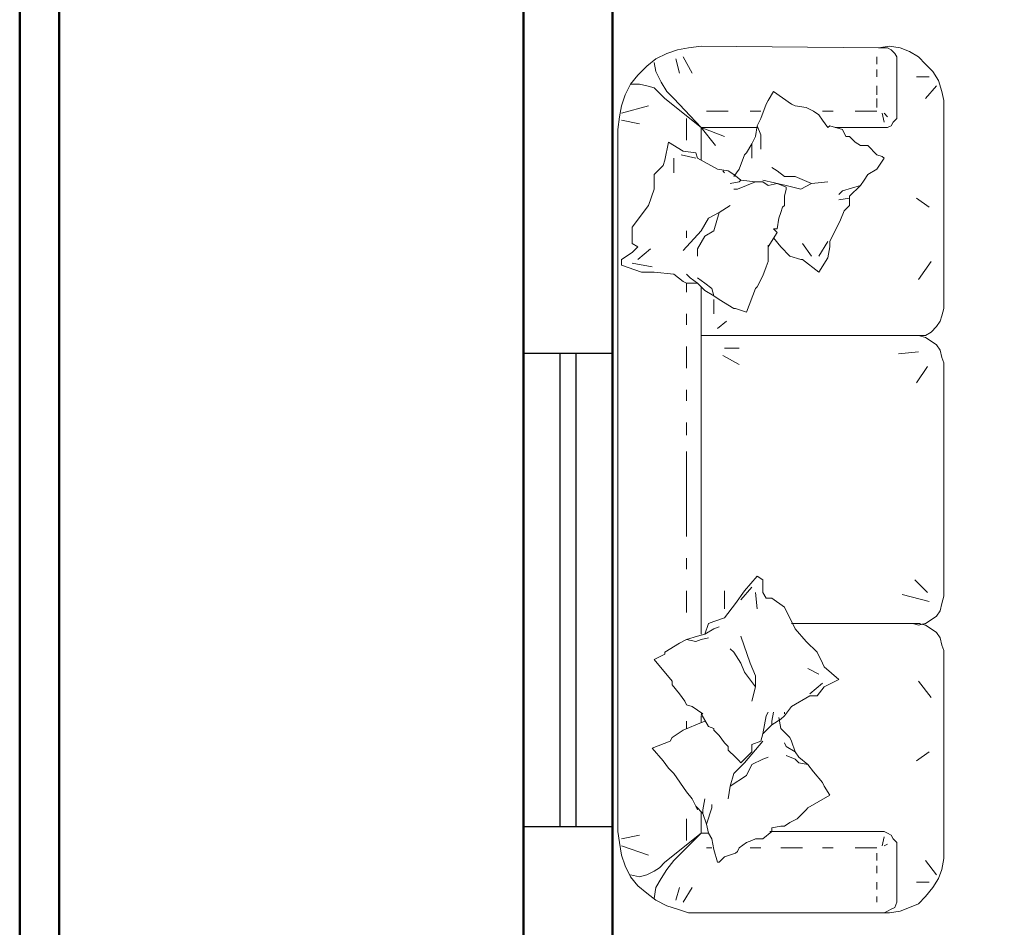
# Model space of a CAD drawing. Units: inches. Extents: x -466983 to 1020, y 324 to 318697.
# Tile 42 of 97: x 392 to 491, y 881 to 973. Entities that reach past the tile are written whole.
import ezdxf

# ---------------------------------------------------------------- set-up
doc = ezdxf.new("R2010")
doc.units = ezdxf.units.IN
doc.header["$MEASUREMENT"] = 0
for name, color, linetype, lineweight in [('A-FLOR-PATT', 252, 'Continuous', 13), ('A-FURN', 8, 'Continuous', 18), ('A-GLAZ', 4, 'Continuous', 25), ('A-WALL', 7, 'Continuous', 50)]:
    doc.layers.add(name, color=color, linetype=linetype, lineweight=lineweight)

# ---------------------------------------------------------------- blocks, each defined once
blk = doc.blocks.new('Window 4 ft')
for p, q in [((1224.69, 893.769), (1233.69, 893.769)), ((1224.69, 845.769), (1224.69, 893.769)), ((1228.39, 845.769), (1228.39, 893.769)), ((1229.99, 893.769), (1229.99, 845.769)), ((1233.69, 893.769), (1233.69, 845.769)), ((1233.69, 845.769), (1224.69, 845.769))]:
    blk.add_line(p, q)
blk = doc.blocks.new('sofa-36')
at = {"linetype": 'ByBlock'}
for p, q in [((-0.105, 0.895), (-0.08, 0.9)), ((-0.08, 0.9), (-0.105, 0.895)), ((-0.08, 0.9), (0.495, 0.9)), ((0.495, 0.9), (-0.08, 0.9)), ((0.495, 0.9), (0.515, 0.895)), ((0.515, 0.895), (0.495, 0.9)), ((0.63, 0.895), (0.645, 0.9)), ((0.63, 0.895), (0.645, 0.9)), ((0.645, 0.9), (0.87, 0.9)), ((0.87, 0.9), (0.645, 0.9)), ((0.87, 0.9), (1.29, 0.9)), ((1.29, 0.9), (0.87, 0.9)), ((1.29, 0.9), (1.31, 0.895)), ((1.31, 0.895), (1.29, 0.9)), ((1.425, 0.895), (1.44, 0.9)), ((1.425, 0.895), (1.44, 0.9)), ((1.44, 0.9), (2.015, 0.9)), ((2.015, 0.9), (1.44, 0.9)), ((2.015, 0.9), (2.045, 0.895)), ((2.045, 0.895), (2.015, 0.9)), ((-0.18, 0.85), (-0.16, 0.87)), ((-0.16, 0.87), (-0.18, 0.85)), ((-0.16, 0.87), (-0.135, 0.885)), ((-0.135, 0.885), (-0.16, 0.87)), ((-0.135, 0.885), (-0.105, 0.895)), ((-0.105, 0.895), (-0.135, 0.885)), ((-0.085, 0.85), (-0.12, 0.88)), ((0.515, 0.895), (0.53, 0.89)), ((0.53, 0.89), (0.515, 0.895)), ((0.53, 0.89), (0.545, 0.88)), ((0.545, 0.88), (0.53, 0.89)), ((0.545, 0.88), (0.56, 0.865)), ((0.56, 0.865), (0.545, 0.88)), ((0.585, 0.865), (0.595, 0.88)), ((0.585, 0.865), (0.595, 0.88)), ((0.595, 0.88), (0.61, 0.89)), ((0.595, 0.88), (0.61, 0.89)), ((0.61, 0.89), (0.63, 0.895)), ((0.61, 0.89), (0.63, 0.895)), ((1.31, 0.895), (1.33, 0.89)), ((1.33, 0.89), (1.31, 0.895)), ((1.33, 0.89), (1.345, 0.88)), ((1.345, 0.88), (1.33, 0.89)), ((1.345, 0.88), (1.355, 0.865)), ((1.355, 0.865), (1.345, 0.88)), ((1.38, 0.865), (1.39, 0.88)), ((1.38, 0.865), (1.39, 0.88)), ((1.39, 0.88), (1.405, 0.89)), ((1.39, 0.88), (1.405, 0.89)), ((1.405, 0.89), (1.425, 0.895)), ((1.405, 0.89), (1.425, 0.895)), ((2.02, 0.85), (2.06, 0.88)), ((2.045, 0.895), (2.07, 0.885)), ((2.07, 0.885), (2.045, 0.895)), ((2.07, 0.885), (2.095, 0.87)), ((2.095, 0.87), (2.07, 0.885)), ((2.095, 0.87), (2.12, 0.85)), ((2.12, 0.85), (2.095, 0.87)), ((-0.2, 0.83), (-0.18, 0.85)), ((-0.18, 0.85), (-0.2, 0.83)), ((-0.145, 0.825), (-0.145, 0.86)), ((0.19, 0.825), (0.215, 0.86)), ((0.415, 0.83), (0.365, 0.865)), ((0.56, 0.865), (0.57, 0.85)), ((0.57, 0.85), (0.56, 0.865)), ((0.57, 0.83), (0.575, 0.85)), ((0.57, 0.85), (0.57, 0.83)), ((0.57, 0.83), (0.57, 0.85)), ((0.57, 0.83), (0.575, 0.85)), ((0.575, 0.85), (0.585, 0.865)), ((0.575, 0.85), (0.585, 0.865)), ((0.655, 0.855), (0.7, 0.825)), ((1.28, 0.855), (1.245, 0.82)), ((1.305, 0.86), (1.285, 0.785)), ((1.355, 0.865), (1.365, 0.85)), ((1.365, 0.85), (1.355, 0.865)), ((1.365, 0.85), (1.3675, 0.84)), ((1.37, 0.83), (1.365, 0.85)), ((1.365, 0.83), (1.37, 0.85)), ((1.3675, 0.84), (1.37, 0.85)), ((1.37, 0.85), (1.38, 0.865)), ((1.37, 0.85), (1.38, 0.865)), ((1.525, 0.83), (1.57, 0.865)), ((1.745, 0.825), (1.72, 0.86)), ((2.08, 0.825), (2.08, 0.86)), ((2.12, 0.85), (2.14, 0.83)), ((2.14, 0.83), (2.12, 0.85)), ((-0.215, 0.805), (-0.2, 0.83)), ((-0.2, 0.83), (-0.215, 0.805)), ((0.57, 0.835), (0.57, 0.23)), ((0.57, 0.815), (0.57, 0.83)), ((0.57, 0.815), (0.57, 0.83)), ((0.615, 0.83), (0.62, 0.775)), ((1.365, 0.835), (1.365, 0.48)), ((1.365, 0.815), (1.37, 0.83)), ((1.365, 0.815), (1.365, 0.83)), ((2.14, 0.83), (2.15, 0.805)), ((2.15, 0.805), (2.14, 0.83)), ((-0.225, 0.78), (-0.215, 0.805)), ((-0.215, 0.805), (-0.225, 0.78)), ((2.15, 0.805), (2.16, 0.78)), ((2.16, 0.78), (2.15, 0.805)), ((-0.23, 0.75), (-0.225, 0.78)), ((-0.225, 0.78), (-0.23, 0.75)), ((-0.22, 0.755), (-0.21, 0.765)), ((-0.21, 0.765), (-0.2, 0.77)), ((-0.2, 0.77), (-0.19, 0.77)), ((-0.19, 0.77), (-0.175, 0.77)), ((-0.175, 0.77), (-0.055, 0.77)), ((-0.055, 0.77), (-0.04, 0.77)), ((-0.04, 0.77), (-0.03, 0.77)), ((-0.03, 0.77), (-0.02, 0.76)), ((1.96, 0.76), (1.97, 0.77)), ((1.97, 0.77), (1.98, 0.77)), ((1.98, 0.77), (1.99, 0.77)), ((1.99, 0.77), (2.115, 0.77)), ((2.115, 0.77), (2.125, 0.77)), ((2.125, 0.77), (2.135, 0.77)), ((2.135, 0.77), (2.15, 0.765)), ((2.15, 0.765), (2.155, 0.755)), ((2.16, 0.78), (2.165, 0.75)), ((2.165, 0.75), (2.16, 0.78)), ((-0.225, 0.72), (-0.23, 0.75)), ((-0.23, 0.75), (-0.225, 0.72)), ((-0.225, 0.745), (-0.22, 0.755)), ((-0.225, 0.735), (-0.225, 0.745)), ((-0.225, 0.72), (-0.225, 0.735)), ((-0.045, 0.735), (-0.035, 0.745)), ((-0.045, 0.73), (-0.02, 0.735)), ((-0.02, 0.76), (-0.01, 0.755)), ((-0.01, 0.755), (-0.005, 0.745)), ((-0.005, 0.745), (-0.005, 0.735)), ((-0.005, 0.735), (-0.005, 0.72)), ((0.08, 0.735), (0.075, 0.73)), ((0.11, 0.715), (0.08, 0.735)), ((1.94, 0.735), (1.945, 0.745)), ((1.94, 0.72), (1.94, 0.735)), ((1.945, 0.745), (1.95, 0.755)), ((1.95, 0.755), (1.96, 0.76)), ((1.98, 0.73), (1.955, 0.735)), ((1.98, 0.735), (1.975, 0.745)), ((2.155, 0.755), (2.16, 0.745)), ((2.16, 0.745), (2.165, 0.735)), ((2.165, 0.75), (2.165, 0.72)), ((2.165, 0.72), (2.165, 0.75)), ((2.165, 0.735), (2.165, 0.72)), ((-0.23, 0.23), (-0.225, 0.72)), ((-0.23, 0.23), (-0.225, 0.72)), ((-0.2, 0.715), (-0.18, 0.715)), ((-0.165, 0.715), (-0.145, 0.715)), ((-0.12, 0.715), (-0.095, 0.715)), ((-0.085, 0.715), (-0.06, 0.715)), ((-0.05, 0.715), (-0.05, 0.655)), ((-0.005, 0.72), (-0.005, 0.6)), ((0.07, 0.715), (0.045, 0.69)), ((0.075, 0.73), (0.07, 0.715)), ((0.125, 0.69), (0.11, 0.715)), ((1.94, 0.42), (1.94, 0.72)), ((1.985, 0.715), (1.985, 0.655)), ((2.02, 0.715), (2, 0.715)), ((2.055, 0.715), (2.035, 0.715)), ((2.1, 0.715), (2.08, 0.715)), ((2.135, 0.715), (2.12, 0.715)), ((2.165, 0.72), (2.165, 0.23)), ((2.165, 0.72), (2.165, 0.23)), ((0.045, 0.69), (0.045, 0.68)), ((0.045, 0.68), (0.045, 0.67)), ((0.14, 0.68), (0.125, 0.69)), ((0.155, 0.67), (0.14, 0.68)), ((0.035, 0.655), (0.02, 0.64)), ((0.045, 0.67), (0.035, 0.655)), ((0.155, 0.67), (0.17, 0.62)), ((0.185, 0.64), (0.155, 0.67)), ((0.02, 0.63), (0, 0.62)), ((0.02, 0.64), (0.02, 0.63)), ((0.185, 0.64), (0.21, 0.64)), ((0.19, 0.64), (0.185, 0.64)), ((0.195, 0.61), (0.19, 0.64)), ((0.21, 0.64), (0.225, 0.625)), ((0, 0.62), (-0.01, 0.585)), ((0.17, 0.62), (0.18, 0.61)), ((0.225, 0.625), (0.25, 0.615)), ((0.235, 0.62), (0.235, 0.62)), ((0.25, 0.615), (0.31, 0.585)), ((1.52, 0.61), (1.485, 0.57)), ((1.54, 0.57), (1.52, 0.61)), ((-0.05, 0.595), (-0.05, 0.565)), ((-0.005, 0.58), (-0.025, 0.565)), ((-0.01, 0.585), (-0.005, 0.58)), ((0.15, 0.535), (0.145, 0.58)), ((0.31, 0.585), (0.325, 0.585)), ((0.35, 0.555), (0.31, 0.58)), ((0.325, 0.585), (0.355, 0.58)), ((0.355, 0.58), (0.395, 0.555)), ((1.815, 0.57), (1.84, 0.585)), ((1.84, 0.585), (1.875, 0.525)), ((1.985, 0.595), (1.985, 0.565)), ((-0.04, 0.555), (-0.05, 0.54)), ((-0.025, 0.565), (-0.04, 0.555)), ((0.395, 0.555), (0.36, 0.51)), ((1.445, 0.55), (1.415, 0.52)), ((1.475, 0.565), (1.445, 0.55)), ((1.485, 0.57), (1.475, 0.565)), ((1.505, 0.555), (1.49, 0.525)), ((1.53, 0.565), (1.56, 0.53)), ((1.565, 0.55), (1.54, 0.57)), ((1.565, 0.53), (1.565, 0.55)), ((1.775, 0.54), (1.805, 0.565)), ((1.805, 0.565), (1.815, 0.57)), ((-0.06, 0.52), (-0.065, 0.49)), ((-0.05, 0.54), (-0.06, 0.52)), ((0.15, 0.535), (0.13, 0.49)), ((0.165, 0.505), (0.15, 0.535)), ((0.35, 0.535), (0.315, 0.51)), ((1.415, 0.52), (1.38, 0.49)), ((1.595, 0.48), (1.565, 0.53)), ((1.735, 0.5), (1.755, 0.525)), ((1.755, 0.525), (1.75, 0.5)), ((1.755, 0.525), (1.775, 0.54)), ((1.875, 0.525), (1.88, 0.52)), ((1.88, 0.52), (1.905, 0.495)), ((-0.065, 0.49), (-0.07, 0.48)), ((0.13, 0.49), (0.13, 0.46)), ((0.155, 0.465), (0.165, 0.505)), ((0.36, 0.505), (0.35, 0.475)), ((0.36, 0.51), (0.36, 0.505)), ((1.38, 0.49), (1.32, 0.46)), ((1.72, 0.49), (1.69, 0.48)), ((1.705, 0.465), (1.72, 0.49)), ((1.72, 0.49), (1.735, 0.5)), ((1.74, 0.49), (1.73, 0.465)), ((1.75, 0.5), (1.74, 0.49)), ((1.905, 0.495), (1.915, 0.475)), ((1.985, 0.45), (1.985, 0.51)), ((-0.07, 0.48), (-0.105, 0.43)), ((0.14, 0.4), (0.155, 0.465)), ((0.16, 0.465), (0.15, 0.44)), ((0.165, 0.465), (0.16, 0.465)), ((0.185, 0.46), (0.165, 0.465)), ((0.35, 0.475), (0.325, 0.45)), ((1.62, 0.46), (1.595, 0.48)), ((1.68, 0.475), (1.655, 0.45)), ((1.69, 0.48), (1.68, 0.475)), ((1.695, 0.46), (1.705, 0.465)), ((1.915, 0.475), (1.925, 0.46)), ((0.115, 0.44), (0.105, 0.425)), ((0.13, 0.46), (0.115, 0.44)), ((0.15, 0.44), (0.155, 0.415)), ((0.21, 0.46), (0.185, 0.46)), ((0.215, 0.455), (0.21, 0.46)), ((0.23, 0.45), (0.215, 0.455)), ((0.245, 0.445), (0.23, 0.45)), ((0.275, 0.44), (0.245, 0.445)), ((0.275, 0.43), (0.275, 0.44)), ((0.285, 0.44), (0.275, 0.43)), ((0.325, 0.415), (0.285, 0.44)), ((0.325, 0.45), (0.3, 0.43)), ((1.32, 0.46), (1.295, 0.425)), ((1.615, 0.46), (1.61, 0.46)), ((1.63, 0.45), (1.62, 0.46)), ((1.655, 0.45), (1.625, 0.445)), ((1.645, 0.425), (1.63, 0.45)), ((1.925, 0.46), (1.925, 0.45)), ((1.925, 0.45), (1.93, 0.425)), ((-0.105, 0.43), (-0.08, 0.415)), ((-0.08, 0.415), (-0.07, 0.41)), ((-0.07, 0.41), (-0.03, 0.395)), ((0.155, 0.415), (0.145, 0.4)), ((0.32, 0.415), (0.325, 0.415)), ((0.355, 0.415), (0.32, 0.415)), ((0.365, 0.415), (0.355, 0.415)), ((0.38, 0.41), (0.365, 0.415)), ((0.405, 0.4), (0.38, 0.41)), ((1.295, 0.41), (1.28, 0.4)), ((1.295, 0.425), (1.295, 0.41)), ((1.61, 0.43), (1.635, 0.425)), ((1.62, 0.41), (1.61, 0.415)), ((1.67, 0.4), (1.62, 0.41)), ((1.635, 0.425), (1.645, 0.425)), ((1.645, 0.425), (1.67, 0.4)), ((1.74, 0.4), (1.735, 0.415)), ((1.93, 0.425), (1.94, 0.425)), ((1.94, 0.425), (1.96, 0.4)), ((-0.05, 0.365), (-0.05, 0.395)), ((-0.03, 0.395), (-0.01, 0.385)), ((-0.01, 0.385), (0.015, 0.395)), ((-0.01, 0.385), (0.02, 0.38)), ((-0.005, 0.385), (-0.005, 0.23)), ((0.015, 0.395), (0.03, 0.395)), ((0.03, 0.395), (0.055, 0.395)), ((0.145, 0.4), (0.145, 0.38)), ((0.435, 0.385), (0.405, 0.4)), ((0.44, 0.38), (0.435, 0.385)), ((1.245, 0.4), (1.235, 0.385)), ((1.235, 0.385), (1.275, 0.35)), ((1.28, 0.4), (1.245, 0.4)), ((1.28, 0.38), (1.325, 0.385)), ((1.67, 0.4), (1.69, 0.395)), ((1.69, 0.4), (1.75, 0.35)), ((1.69, 0.395), (1.7, 0.37)), ((1.755, 0.37), (1.74, 0.4)), ((1.96, 0.4), (1.96, 0.38)), ((1.985, 0.365), (1.985, 0.395)), ((0.02, 0.38), (0.04, 0.37)), ((0.04, 0.37), (0.065, 0.355)), ((0.04, 0.37), (0.065, 0.37)), ((0.065, 0.37), (0.08, 0.37)), ((0.065, 0.355), (0.07, 0.35)), ((0.145, 0.38), (0.14, 0.34)), ((0.145, 0.38), (0.165, 0.33)), ((0.505, 0.355), (0.44, 0.38)), ((0.495, 0.325), (0.505, 0.355)), ((1.265, 0.37), (1.3, 0.34)), ((1.4, 0.34), (1.475, 0.365)), ((1.475, 0.365), (1.51, 0.38)), ((1.54, 0.38), (1.5, 0.35)), ((1.51, 0.38), (1.54, 0.38)), ((1.54, 0.38), (1.58, 0.37)), ((1.7, 0.37), (1.72, 0.37)), ((1.72, 0.37), (1.75, 0.34)), ((1.785, 0.355), (1.755, 0.37)), ((1.815, 0.31), (1.785, 0.355)), ((1.96, 0.38), (1.965, 0.37)), ((1.965, 0.37), (1.97, 0.355)), ((1.97, 0.355), (1.985, 0.335)), ((0.07, 0.35), (0.11, 0.335)), ((0.11, 0.335), (0.13, 0.32)), ((0.14, 0.34), (0.125, 0.32)), ((0.14, 0.34), (0.145, 0.335)), ((0.145, 0.335), (0.15, 0.31)), ((0.165, 0.33), (0.165, 0.32)), ((0.605, 0.295), (0.605, 0.335)), ((0.625, 0.29), (0.65, 0.335)), ((1.275, 0.35), (1.31, 0.325)), ((1.475, 0.34), (1.445, 0.32)), ((1.5, 0.35), (1.475, 0.34)), ((1.745, 0.335), (1.735, 0.325)), ((1.75, 0.34), (1.745, 0.335)), ((1.75, 0.35), (1.78, 0.32)), ((1.985, 0.335), (1.995, 0.33)), ((1.995, 0.33), (2, 0.325)), ((-0.05, 0.245), (-0.05, 0.305)), ((0.115, 0.305), (0.11, 0.275)), ((0.125, 0.32), (0.115, 0.305)), ((0.23, 0.28), (0.21, 0.31)), ((0.47, 0.28), (0.495, 0.32)), ((0.495, 0.32), (0.495, 0.325)), ((0.55, 0.275), (0.53, 0.3)), ((1.31, 0.325), (1.35, 0.295)), ((1.445, 0.32), (1.435, 0.31)), ((1.705, 0.305), (1.695, 0.295)), ((1.715, 0.305), (1.705, 0.305)), ((1.735, 0.325), (1.715, 0.305)), ((1.78, 0.32), (1.815, 0.31)), ((1.815, 0.31), (1.85, 0.305)), ((2, 0.325), (2.01, 0.295)), ((0.02, 0.295), (-0.005, 0.23)), ((0.11, 0.275), (0.08, 0.22)), ((0.12, 0.295), (0.115, 0.29)), ((0.23, 0.28), (0.28, 0.265)), ((0.245, 0.25), (0.23, 0.28)), ((0.46, 0.265), (0.47, 0.28)), ((1.325, 0.295), (1.275, 0.295)), ((1.35, 0.295), (1.36, 0.265)), ((1.38, 0.265), (1.375, 0.28)), ((1.675, 0.28), (1.66, 0.265)), ((1.695, 0.295), (1.675, 0.28)), ((2.025, 0.275), (1.99, 0.265)), ((2.01, 0.295), (2.025, 0.28)), ((2.025, 0.28), (2.025, 0.275)), ((0.045, 0.27), (-0.005, 0.23)), ((0.28, 0.23), (0.245, 0.25)), ((0.28, 0.265), (0.295, 0.24)), ((0.425, 0.24), (0.44, 0.26)), ((0.44, 0.26), (0.46, 0.265)), ((0.445, 0.24), (0.46, 0.265)), ((0.51, 0.265), (0.47, 0.265)), ((1.36, 0.265), (1.365, 0.25)), ((1.365, 0.25), (1.395, 0.24)), ((1.395, 0.24), (1.38, 0.265)), ((1.41, 0.23), (1.405, 0.25)), ((1.65, 0.25), (1.615, 0.23)), ((1.655, 0.265), (1.65, 0.25)), ((1.66, 0.265), (1.655, 0.265)), ((1.875, 0.26), (1.865, 0.26)), ((1.92, 0.245), (1.875, 0.26)), ((1.92, 0.245), (1.89, 0.235)), ((1.945, 0.25), (1.92, 0.245)), ((1.96, 0.26), (1.945, 0.25)), ((1.945, 0.25), (1.945, 0.23)), ((1.99, 0.265), (1.96, 0.26)), ((1.985, 0.245), (1.985, 0.26)), ((-0.225, 0.195), (-0.23, 0.23)), ((-0.225, 0.195), (-0.23, 0.23)), ((-0.005, 0.23), (-0.085, 0.13)), ((-0.005, 0.23), (-0.085, 0.155)), ((0.085, 0.23), (-0.005, 0.23)), ((0.08, 0.22), (0.065, 0.215)), ((0.335, 0.18), (0.28, 0.23)), ((0.295, 0.24), (0.33, 0.22)), ((0.33, 0.22), (0.35, 0.22)), ((0.41, 0.22), (0.425, 0.24)), ((0.425, 0.22), (0.41, 0.2)), ((0.425, 0.22), (0.445, 0.24)), ((0.425, 0.19), (0.425, 0.22)), ((0.435, 0.23), (0.87, 0.23)), ((1.395, 0.23), (0.87, 0.23)), ((1.4, 0.22), (1.395, 0.24)), ((1.41, 0.19), (1.4, 0.22)), ((1.415, 0.215), (1.41, 0.23)), ((1.615, 0.235), (1.595, 0.205)), ((1.615, 0.23), (1.615, 0.235)), ((1.615, 0.23), (1.615, 0.23)), ((1.64, 0.23), (1.62, 0.23)), ((1.645, 0.215), (1.635, 0.24)), ((1.88, 0.235), (1.85, 0.24)), ((1.89, 0.235), (1.87, 0.215)), ((1.87, 0.215), (1.88, 0.22)), ((1.89, 0.235), (1.88, 0.235)), ((1.885, 0.23), (1.945, 0.23)), ((1.945, 0.23), (2.025, 0.13)), ((1.945, 0.23), (2.02, 0.155)), ((2.165, 0.23), (2.165, 0.195)), ((2.165, 0.23), (2.165, 0.195)), ((-0.22, 0.165), (-0.225, 0.195)), ((-0.22, 0.165), (-0.225, 0.195)), ((-0.2, 0.18), (-0.155, 0.205)), ((0.065, 0.215), (0.06, 0.18)), ((0.07, 0.175), (0.08, 0.215)), ((0.41, 0.2), (0.4, 0.19)), ((1.41, 0.19), (1.415, 0.215)), ((1.595, 0.205), (1.59, 0.19)), ((1.66, 0.18), (1.645, 0.215)), ((1.85, 0.205), (1.83, 0.19)), ((1.845, 0.2), (1.845, 0.2)), ((1.87, 0.215), (1.85, 0.205)), ((2.135, 0.18), (2.095, 0.205)), ((2.165, 0.195), (2.155, 0.165)), ((2.165, 0.195), (2.155, 0.165)), ((-0.21, 0.135), (-0.22, 0.165)), ((-0.21, 0.135), (-0.22, 0.165)), ((-0.155, 0.17), (-0.195, 0.16)), ((-0.03, 0.19), (0.03, 0.19)), ((0.06, 0.18), (0.035, 0.14)), ((0.28, 0.19), (0.3, 0.19)), ((0.4, 0.155), (0.42, 0.18)), ((0.42, 0.18), (0.425, 0.19)), ((0.45, 0.19), (0.425, 0.19)), ((0.54, 0.19), (0.51, 0.19)), ((0.6, 0.19), (0.66, 0.19)), ((0.72, 0.19), (0.75, 0.19)), ((0.81, 0.19), (0.845, 0.19)), ((1.125, 0.19), (0.89, 0.19)), ((1.215, 0.19), (1.185, 0.19)), ((1.335, 0.19), (1.275, 0.19)), ((1.42, 0.17), (1.41, 0.19)), ((1.445, 0.13), (1.42, 0.17)), ((1.56, 0.17), (1.535, 0.15)), ((1.58, 0.185), (1.56, 0.17)), ((1.59, 0.19), (1.58, 0.185)), ((1.655, 0.19), (1.635, 0.19)), ((1.68, 0.15), (1.66, 0.18)), ((1.83, 0.19), (1.78, 0.155)), ((1.965, 0.19), (1.905, 0.19)), ((2.095, 0.17), (2.13, 0.16)), ((2.155, 0.165), (2.145, 0.135)), ((2.155, 0.165), (2.145, 0.135)), ((-0.085, 0.155), (-0.105, 0.135)), ((0.035, 0.14), (0.085, 0.13)), ((0.08, 0.155), (0.12, 0.155)), ((0.395, 0.1), (0.4, 0.155)), ((1.525, 0.15), (1.465, 0.1)), ((1.535, 0.15), (1.525, 0.15)), ((1.69, 0.145), (1.68, 0.15)), ((1.71, 0.095), (1.69, 0.145)), ((1.765, 0.14), (1.745, 0.125)), ((1.78, 0.155), (1.765, 0.14)), ((2.02, 0.155), (2.045, 0.135)), ((-0.195, 0.105), (-0.21, 0.135)), ((-0.195, 0.105), (-0.21, 0.135)), ((-0.13, 0.12), (-0.16, 0.105)), ((-0.105, 0.135), (-0.13, 0.12)), ((-0.1, 0.115), (-0.115, 0.1)), ((-0.085, 0.13), (-0.1, 0.115)), ((0.085, 0.13), (0.1, 0.125)), ((0.1, 0.125), (0.125, 0.1)), ((1.45, 0.13), (1.445, 0.13)), ((1.465, 0.1), (1.45, 0.13)), ((1.745, 0.125), (1.71, 0.095)), ((2.025, 0.13), (2.04, 0.115)), ((2.04, 0.115), (2.05, 0.1)), ((2.045, 0.135), (2.07, 0.12)), ((2.07, 0.12), (2.095, 0.105)), ((2.145, 0.135), (2.13, 0.105)), ((2.145, 0.135), (2.13, 0.105)), ((-0.175, 0.08), (-0.195, 0.105)), ((-0.175, 0.08), (-0.195, 0.105)), ((-0.16, 0.105), (-0.185, 0.1)), ((-0.115, 0.1), (-0.12, 0.08)), ((-0.045, 0.01), (-0.065, 0.085)), ((0.125, 0.1), (0.165, 0.1)), ((0.165, 0.1), (0.21, 0.085)), ((0.21, 0.085), (0.27, 0.04)), ((0.36, 0.055), (0.33, 0.09)), ((0.37, 0.04), (0.38, 0.095)), ((0.395, 0.065), (0.395, 0.1)), ((1.98, 0.01), (2.005, 0.085)), ((2.05, 0.1), (2.06, 0.08)), ((2.095, 0.105), (2.125, 0.1)), ((2.13, 0.105), (2.11, 0.08)), ((2.13, 0.105), (2.11, 0.08)), ((-0.15, 0.055), (-0.175, 0.08)), ((-0.15, 0.055), (-0.175, 0.08)), ((-0.125, 0.035), (-0.15, 0.055)), ((-0.125, 0.035), (-0.15, 0.055)), ((-0.12, 0.08), (-0.125, 0.06)), ((-0.125, 0.06), (-0.125, 0.035)), ((-0.015, 0.06), (-0.025, 0.01)), ((0.315, 0.04), (0.325, 0.055)), ((0.325, 0.055), (0.34, 0.04)), ((0.375, 0.01), (0.395, 0.065)), ((1.95, 0.06), (1.96, 0.01)), ((2.06, 0.08), (2.065, 0.06)), ((2.065, 0.06), (2.06, 0.035)), ((2.09, 0.055), (2.065, 0.035)), ((2.09, 0.055), (2.065, 0.035)), ((2.11, 0.08), (2.09, 0.055)), ((2.11, 0.08), (2.09, 0.055)), ((-0.095, 0.02), (-0.125, 0.035)), ((-0.095, 0.02), (-0.125, 0.035)), ((0.27, 0.04), (0.315, 0.04)), ((0.34, 0.04), (0.36, 0.01)), ((2.065, 0.035), (2.035, 0.02)), ((2.065, 0.035), (2.035, 0.02)), ((-0.065, 0.01), (-0.095, 0.02)), ((-0.065, 0.01), (-0.095, 0.02)), ((-0.035, 0.005), (-0.065, 0.01)), ((-0.035, 0.005), (-0.065, 0.01)), ((0, 0), (-0.035, 0.005)), ((0, 0), (-0.035, 0.005)), ((1.94, 0), (0, 0)), ((1.94, 0), (0, 0)), ((0.36, 0.01), (0.375, 0.01)), ((1.97, 0.005), (1.94, 0)), ((1.97, 0.005), (1.94, 0)), ((2.005, 0.01), (1.97, 0.005)), ((2.005, 0.01), (1.97, 0.005)), ((2.035, 0.02), (2.005, 0.01)), ((2.035, 0.02), (2.005, 0.01))]:
    blk.add_line(p, q, dxfattribs=at)

msp = doc.modelspace()

# ---------------------------------------------------------------- hatches: boundary and pattern name
at = {"layer": 'A-FLOR-PATT', "transparency": 33554572}
h = msp.add_hatch(dxfattribs=at)
h.set_pattern_fill('ANSI37', color=256, scale=30)
h.set_pattern_definition([(45, (-1212.4137, -290.035), (-2.6516504, 2.6516504), []), (135, (-1212.4137, -290.035), (-2.6516504, -2.6516504), [])])
h.paths.add_polyline_path([(901.806, 1075.938), (900.614, 1075.938), (900.614, 1065.386), (899.391, 1065.386), (898.091, 1065.386), (892.836, 1058.71, -0.258377), (892.188, 1058.351), (879.985, 1058.351, -0.20177), (879.438, 1058.581), (874.081, 1065.386), (872.781, 1065.386), (871.558, 1065.386), (871.558, 1075.938), (813.806, 1075.938), (813.806, 1044.792), (832.395, 1044.792, -0.394795), (848.66, 1028.536), (848.66, 1009.938), (901.806, 1009.938), (901.806, 1015.938), (901.306, 1015.938), (871.306, 1015.938), (871.306, 1017.25), (871.334, 1017.25, -0.401453), (901.306, 1045.938), (901.806, 1045.938)])
edge = h.paths.add_edge_path(flags=16)
edge.add_line((847.773, 1068.949), (847.773, 1073.709))
edge.add_arc((849.227, 1073.709), 1.454, 90, 180, ccw=False)
edge.add_line((849.227, 1075.163), (864.492, 1075.163))
edge.add_arc((864.492, 1073.709), 1.454, 0, 90, ccw=False)
edge.add_line((865.946, 1073.709), (865.946, 1069.004))
edge.add_arc((832.645, 1068.976), 33.301, -20.61234, 0.04725, ccw=False)
edge.add_ellipse((856.859, 1058.48), major_axis=(0, 10.213), ratio=0.685919, start_angle=100.00884, end_angle=259.99116, ccw=False)
edge.add_arc((881.074, 1068.976), 33.301, 180.04725, 200.61234, ccw=False)
h.paths.add_polyline_path([(853.146, 1066.482), (853.146, 1066.453), (853.146, 1066.453, 0.433107), (852.917, 1066.685), (852.917, 1066.453), (853.146, 1066.453), (853.146, 1066.482), (853.088, 1066.612, 0.697939), (852.7, 1066.453), (852.7, 1066.453), (852.7, 1066.482), (852.917, 1067.001), (852.917, 1066.685, -0.396254)], flags=0)
h.paths.add_polyline_path([(861.019, 1066.482), (861.019, 1066.453), (861.019, 1066.453, 0.416404), (860.802, 1066.685), (860.802, 1066.453), (861.019, 1066.453), (861.019, 1066.482), (860.967, 1066.605, 0.713344), (860.573, 1066.453), (860.573, 1066.453), (860.573, 1066.482), (860.802, 1067.001), (860.802, 1066.685, -0.379973)], flags=0)
edge = h.paths.add_edge_path(flags=0)
edge.add_spline(control_points=[(861.13, 1065.785), (861.466, 1065.248), (861.613, 1065.016), (861.983, 1064.374), (862.192, 1063.944), (862.561, 1063.039), (862.721, 1062.563), (862.987, 1061.578), (863.092, 1061.069), (863.245, 1060.031), (863.293, 1059.503), (863.329, 1058.441), (863.318, 1057.908), (863.237, 1056.852), (863.166, 1056.329), (862.97, 1055.308), (862.843, 1054.81), (862.537, 1053.852), (862.357, 1053.393), (861.951, 1052.525), (861.725, 1052.117), (861.233, 1051.362), (860.967, 1051.016), (860.405, 1050.395), (860.108, 1050.12), (859.494, 1049.646), (859.176, 1049.448), (858.528, 1049.13), (858.197, 1049.011), (857.531, 1048.852), (857.196, 1048.812), (856.525, 1048.812), (856.189, 1048.852), (855.524, 1049.01), (855.193, 1049.129), (854.545, 1049.447), (854.227, 1049.645), (853.612, 1050.118), (853.316, 1050.393), (852.753, 1051.014), (852.487, 1051.36), (851.995, 1052.114), (851.769, 1052.523), (851.363, 1053.39), (851.183, 1053.85), (850.877, 1054.807), (850.75, 1055.305), (850.553, 1056.326), (850.483, 1056.849), (850.401, 1057.905), (850.39, 1058.438), (850.426, 1059.5), (850.473, 1060.028), (850.626, 1061.066), (850.732, 1061.575), (850.997, 1062.561), (851.157, 1063.036), (851.525, 1063.942), (851.734, 1064.371), (852.106, 1065.016), (852.254, 1065.25), (852.608, 1065.733)], knot_values=[3.915332, 3.915332, 3.915332, 3.915332, 4.013468, 4.013468, 4.175532, 4.175532, 4.337596, 4.337596, 4.49966, 4.49966, 4.661724, 4.661724, 4.823788, 4.823788, 4.985852, 4.985852, 5.147916, 5.147916, 5.30998, 5.30998, 5.472044, 5.472044, 5.634109, 5.634109, 5.796173, 5.796173, 5.958237, 5.958237, 6.120301, 6.120301, 6.282365, 6.282365, 6.444429, 6.444429, 6.606493, 6.606493, 6.768557, 6.768557, 6.930621, 6.930621, 7.092685, 7.092685, 7.254749, 7.254749, 7.416813, 7.416813, 7.578878, 7.578878, 7.740942, 7.740942, 7.903006, 7.903006, 8.06507, 8.06507, 8.227134, 8.227134, 8.389198, 8.389198, 8.551262, 8.551262, 8.65037, 8.65037, 8.65037, 8.65037], degree=3, periodic=0)
edge.add_line((852.642, 1065.785), (861.13, 1065.785))
edge = h.paths.add_edge_path(flags=0)
edge.add_ellipse((856.85, 1057.743), major_axis=(0, 7.792), ratio=0.687861, start_angle=0, end_angle=360)
h.paths.add_polyline_path([(848.863, 1069.389), (848.863, 1073.96, -0.414214), (849.954, 1075.051), (863.765, 1075.051, -0.414214), (864.856, 1073.96), (864.856, 1069.389, -0.388936), (864.524, 1069.027, -0.043561), (849.195, 1069.027, -0.388936)], flags=0)
h.paths.add_polyline_path([(853.101, 1068.112, -1), (852.677, 1068.112, -1)], flags=0)
edge = h.paths.add_edge_path(flags=0)
edge.add_ellipse((856.859, 1057.338), major_axis=(0, 2.207), ratio=0.657164, start_angle=0, end_angle=360)
h.paths.add_polyline_path([(861.041, 1068.112, -1), (860.618, 1068.112, -1)], flags=0)
edge = h.paths.add_edge_path()
edge.add_line((573.954, 1057.341), (573.954, 1075.938))
edge.add_line((573.954, 1075.938), (558.731, 1075.938))
edge.add_line((558.731, 1075.938), (558.731, 1065.386))
edge.add_line((558.731, 1065.386), (557.507, 1065.386))
edge.add_line((557.507, 1065.386), (556.207, 1065.386))
edge.add_line((556.207, 1065.386), (550.952, 1058.71))
edge.add_arc((550.304, 1059.116), 0.765, 270, 327.94832, ccw=False)
edge.add_line((550.304, 1058.351), (538.101, 1058.351))
edge.add_arc((538.101, 1059.116), 0.765, 224.3704, 270, ccw=False)
edge.add_line((537.555, 1058.581), (532.198, 1065.386))
edge.add_line((532.198, 1065.386), (530.898, 1065.386))
edge.add_line((530.898, 1065.386), (529.674, 1065.386))
edge.add_line((529.674, 1065.386), (529.674, 1075.938))
edge.add_line((529.674, 1075.938), (520.806, 1075.938))
edge.add_line((520.806, 1075.938), (520.806, 1045.938))
edge.add_line((520.806, 1045.938), (521.306, 1045.938))
edge.add_arc((521.306, 1015.938), 30, 2.50749, 90, ccw=False)
edge.add_line((551.277, 1017.25), (551.306, 1017.25))
edge.add_line((551.306, 1017.25), (551.306, 1015.938))
edge.add_line((551.306, 1015.938), (520.806, 1015.938))
edge.add_line((520.806, 1015.938), (520.806, 1009.938))
edge.add_line((520.806, 1009.938), (559.191, 1010.402))
edge.add_arc((559.191, 1011.856), 1.454, 180, 270, ccw=False)
edge.add_line((557.737, 1011.856), (557.737, 1016.561))
edge.add_arc((591.039, 1016.589), 33.301, 159.38766, 180.04725, ccw=False)
edge.add_ellipse((566.824, 1027.085), major_axis=(0, 10.213), ratio=0.685919, start_angle=280.00884, end_angle=439.99116, ccw=False)
edge.add_arc((542.609, 1016.589), 33.301, 0.04725, 20.61234, ccw=False)
edge.add_line((575.91, 1016.616), (575.91, 1011.856))
edge.add_arc((574.456, 1011.856), 1.454, -90, 0, ccw=False)
edge.add_line((574.456, 1010.402), (608.806, 1009.938))
edge.add_line((608.806, 1009.938), (608.806, 1041.086))
edge.add_line((608.806, 1041.086), (590.218, 1041.086))
edge.add_arc((590.775, 1057.907), 16.831, 181.92775, 268.10321, ccw=False)
edge = h.paths.add_edge_path()
edge.add_ellipse((494.244, 583.62), major_axis=(0, 10.213), ratio=0.685919, start_angle=280.00884, end_angle=439.99116, ccw=False)
edge.add_arc((470.03, 573.124), 33.301, 0.04725, 20.61234, ccw=False)
edge.add_line((503.331, 573.152), (503.331, 568.392))
edge.add_arc((501.877, 568.392), 1.454, -90, 0, ccw=False)
edge.add_line((501.877, 566.938), (539.806, 566.938))
edge.add_line((539.806, 566.938), (539.806, 572.938))
edge.add_line((539.806, 572.938), (539.306, 572.938))
edge.add_line((539.306, 572.938), (509.306, 572.938))
edge.add_line((509.306, 572.938), (509.306, 574.25))
edge.add_line((509.306, 574.25), (509.334, 574.25))
edge.add_arc((539.306, 572.938), 30, 90, 177.49251, ccw=False)
edge.add_line((539.306, 602.938), (539.806, 602.938))
edge.add_line((539.806, 602.938), (539.806, 626.938))
edge.add_line((539.806, 626.938), (531.772, 626.938))
edge.add_line((531.772, 626.938), (531.772, 616.386))
edge.add_line((531.772, 616.386), (530.548, 616.386))
edge.add_line((530.548, 616.386), (529.249, 616.386))
edge.add_line((529.249, 616.386), (523.711, 609.351))
edge.add_line((523.711, 609.351), (510.777, 609.351))
edge.add_line((510.777, 609.351), (505.239, 616.386))
edge.add_line((505.239, 616.386), (503.939, 616.386))
edge.add_line((503.939, 616.386), (502.715, 616.386))
edge.add_line((502.715, 616.386), (502.715, 626.938))
edge.add_line((502.715, 626.938), (481.698, 626.938))
edge.add_line((481.698, 626.938), (481.698, 610.995))
edge.add_arc((467.27, 611.473), 14.436, 271.92775, 358.10321, ccw=False)
edge.add_line((467.756, 597.045), (451.806, 597.045))
edge.add_line((451.806, 597.045), (451.806, 584.404))
edge.add_line((451.806, 584.404), (451.806, 566.938))
edge.add_line((451.806, 566.938), (486.612, 566.938))
edge.add_arc((486.612, 568.392), 1.454, 180, 270, ccw=False)
edge.add_line((485.158, 568.392), (485.158, 573.097))
edge.add_arc((518.459, 573.124), 33.301, 159.38766, 180.04725, ccw=False)
h.paths.add_polyline_path([(836.261, 1020.733), (879.89, 1020.733), (879.89, 1039.39), (836.261, 1039.39)], flags=25)
h.paths.add_polyline_path([(549.985, 1036.749), (593.614, 1036.749), (593.614, 1055.407), (549.985, 1055.407)], flags=24)
h.paths.add_polyline_path([(475.123, 595.596), (518.752, 595.596), (518.752, 614.253), (475.123, 614.253)], flags=24)

# ---------------------------------------------------------------- linework, layer by layer
at = {"layer": 'A-WALL'}
for p, q in [((391.806, 364.938), (391.806, 1084.938)), ((442.806, 415.938), (442.806, 1084.938)), ((395.806, 368.938), (395.806, 1080.938)), ((451.806, 828.938), (451.806, 1075.938))]:
    msp.add_line(p, q, dxfattribs=at)

# ---------------------------------------------------------------- block references
at = {"layer": 'A-FURN', "xscale": 36.66436083614781, "yscale": 36.66436083614781, "zscale": 36.66436083614781, "rotation": 270}
msp.add_blockref('sofa-36', (452.356, 961.663), dxfattribs=at)
at = {"layer": 'A-GLAZ'}
msp.add_blockref('Window 4 ft', (-781.884, 45.223), dxfattribs=at)

doc.saveas('drawing.dxf')
